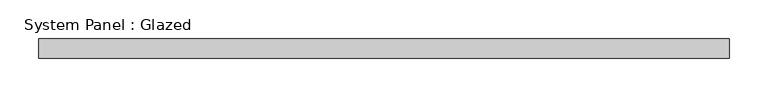
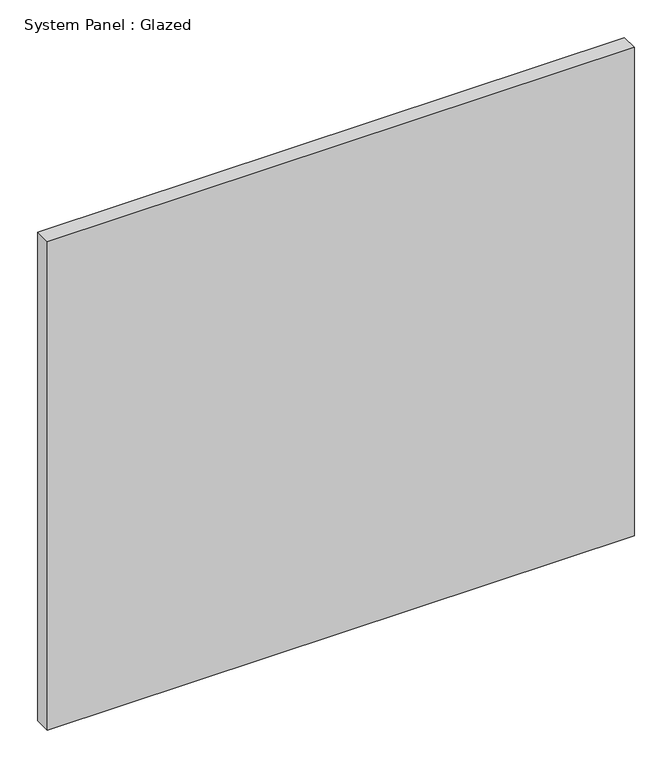
"""IFC4 building model written with IfcOpenShell, lengths in millimetres: plate geometry, System Panel : Glazed."""

from ifc_helpers import new_model, si_unit, origin, origin_with_axes, place, context, project, spatial, polyline, outline, extrude, source, transform, mapped, element, save


def system_panel_glazed_d4207c9f(model_context):
    return source(origin(), model_context, "Body", "SweptSolid", [
        extrude(outline(polyline([(447.675, 19.05), (-447.675, 19.05), (-447.675, 44.45), (447.675, 44.45), (447.675, 19.05)])), origin_with_axes(), (0.0, 0.0, 1.0), 787.4),
    ])


if __name__ == "__main__":
    model = new_model("IFC4")
    model_context = context("Model", 3, world=origin())
    ifc_project = project(units=[si_unit("LENGTHUNIT", "METRE", prefix="MILLI")], contexts=[model_context])
    site = spatial("IfcSite", under=ifc_project)
    building = spatial("IfcBuilding", under=site)
    placement = place(None, origin())
    system_panel_glazed_shape = system_panel_glazed_d4207c9f(model_context)
    element("IfcPlate", 1, ObjectType="System Panel : Glazed", at=placement, inside=building, context=model_context, shape_type="MappedRepresentation", body=[
        mapped(system_panel_glazed_shape, transform((0.0, 0.0, 0.0), x_axis=(1.0, 0.0, 0.0), y_axis=(0.0, 1.0, 0.0), z_axis=(0.0, 0.0, 1.0))),
    ])
    save(model, "model.ifc")

# Revit data of these elements
# Type "System Panel : Glazed"
#   Construction Type Id = "GSP4R"
#   Analytic Construction = "1/8 in Pilkington single glazing"
#   Visual Light Transmittance = 0.9
#   Solar Heat Gain Coefficient = 0.86
#   Heat Transfer Coefficient (U) = 1.18115 BTU/(h·ft²·°F)
#   Define Thermal Properties by = 1
# Element 1 (IfcPlate, "System Panel : Glazed")
#   Materials on its faces: "Glass"
# Materials
#   "Glass": class "Glass", colour RGB 0 128 192, transparency 0.75, Description = "Soda Lime Glass", Cost = 0
